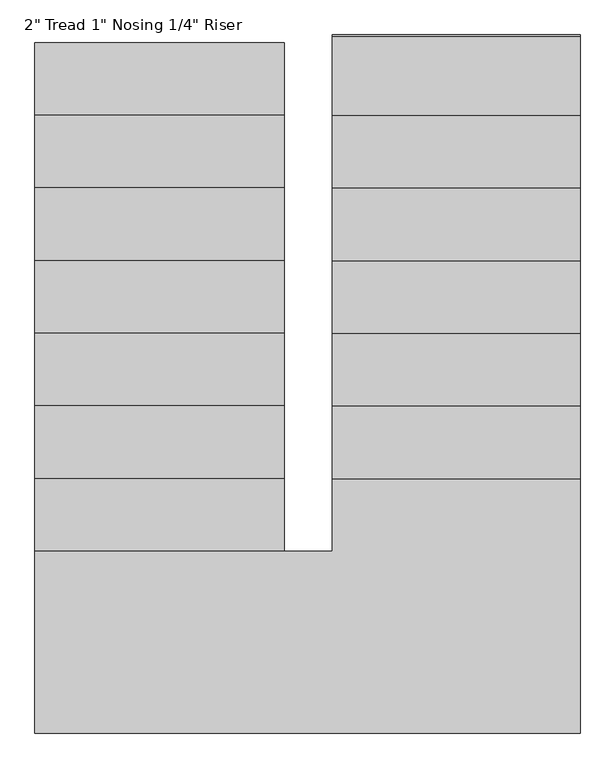
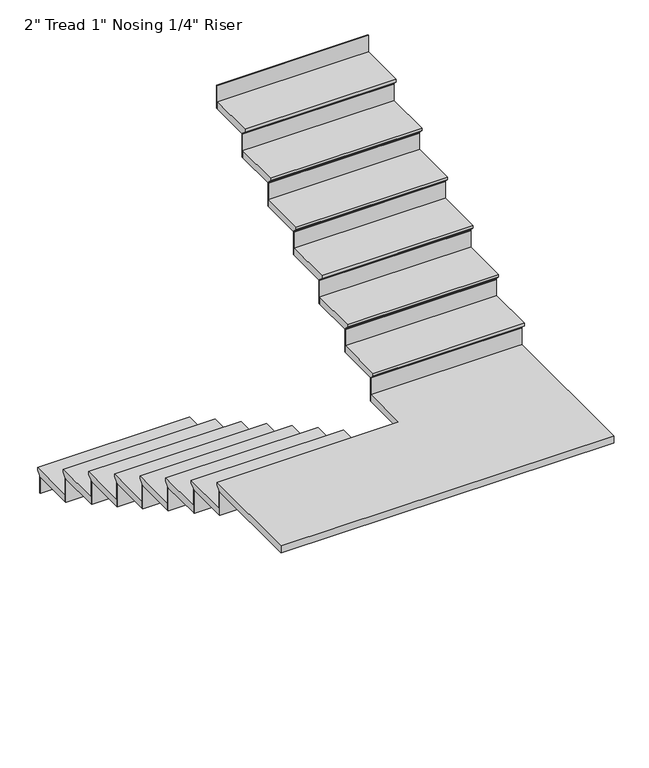
"""IFC4 building model written with IfcOpenShell, lengths in millimetres: stair flight geometry."""

from ifc_helpers import new_model, si_unit, origin, place, context, project, spatial, faceted_brep, source, transform, mapped, element, save


def stair_flight_bd25c6f5(model_context):
    return source(origin(), model_context, "Body", "Brep", [
        faceted_brep([(-4232.280864, -3571.6080018, 12799.4833333), (-4232.280864, -3571.6080018, 12818.5333333), (-3187.6083919, -3571.6080018, 12818.5333333), (-3187.6083919, -3571.6080018, 12799.4833333), (-4232.280864, -3597.0080018, 12774.0833333), (-3187.6083919, -3597.0080018, 12774.0833333), (-4232.280864, -3901.8080018, 12818.5333333), (-3187.6083919, -3901.8080018, 12818.5333333), (-3187.6083919, -3597.0080018, 12767.7333333), (-3187.6083919, -3901.8080018, 12767.7333333), (-4232.280864, -3901.8080018, 12767.7333333), (-4232.280864, -3597.0080018, 12767.7333333)], [[[0, 1, 2, 3]], [[4, 0, 3, 5]], [[2, 1, 6, 7]], [[8, 9, 10, 11]], [[2, 7, 9, 8, 5, 3]], [[8, 11, 4, 5]], [[6, 1, 0, 4, 11, 10]], [[7, 6, 10, 9]]]),
        faceted_brep([(-4232.280864, -3597.0080018, 12767.7333333), (-4232.280864, -3597.0080018, 12649.2), (-4232.280864, -3603.3580018, 12649.2), (-4232.280864, -3603.3580018, 12767.7333333), (-3187.6083919, -3597.0080018, 12767.7333333), (-3187.6083919, -3603.3580018, 12767.7333333), (-3187.6083919, -3603.3580018, 12649.2), (-3187.6083919, -3597.0080018, 12649.2)], [[[0, 1, 2, 3]], [[4, 5, 6, 7]], [[1, 0, 4, 7]], [[2, 1, 7, 6]], [[3, 2, 6, 5]], [[0, 3, 5, 4]]]),
        faceted_brep([(-4232.280864, -3901.8080018, 12937.0666667), (-4232.280864, -3901.8080018, 12767.7333333), (-4232.280864, -3908.1580018, 12767.7333333), (-4232.280864, -3908.1580018, 12937.0666667), (-3187.6083919, -3901.8080018, 12937.0666667), (-3187.6083919, -3908.1580018, 12937.0666667), (-3187.6083919, -3908.1580018, 12767.7333333), (-3187.6083919, -3901.8080018, 12767.7333333)], [[[0, 1, 2, 3]], [[4, 5, 6, 7]], [[1, 0, 4, 7]], [[2, 1, 7, 6]], [[3, 2, 6, 5]], [[0, 3, 5, 4]]]),
        faceted_brep([(-3187.6083919, -3876.4080018, 12987.8666667), (-4232.280864, -3876.4080018, 12987.8666667), (-4232.280864, -4206.6080018, 12987.8666667), (-3187.6083919, -4206.6080018, 12987.8666667), (-3187.6083919, -3901.8080018, 12937.0666667), (-3187.6083919, -4206.6080018, 12937.0666667), (-4232.280864, -4206.6080018, 12937.0666667), (-4232.280864, -3901.8080018, 12937.0666667), (-3187.6083919, -3901.8080018, 12943.4166667), (-3187.6083919, -3876.4080018, 12968.8166667), (-4232.280864, -3901.8080018, 12943.4166667), (-4232.280864, -3876.4080018, 12968.8166667)], [[[0, 1, 2, 3]], [[4, 5, 6, 7]], [[0, 3, 5, 4, 8, 9]], [[4, 7, 10, 8]], [[2, 1, 11, 10, 7, 6]], [[3, 2, 6, 5]], [[11, 1, 0, 9]], [[10, 11, 9, 8]]]),
        faceted_brep([(-4232.280864, -4206.6080018, 13106.4), (-4232.280864, -4206.6080018, 12937.0666667), (-4232.280864, -4212.9580018, 12937.0666667), (-4232.280864, -4212.9580018, 13106.4), (-3187.6083919, -4206.6080018, 13106.4), (-3187.6083919, -4212.9580018, 13106.4), (-3187.6083919, -4212.9580018, 12937.0666667), (-3187.6083919, -4206.6080018, 12937.0666667)], [[[0, 1, 2, 3]], [[4, 5, 6, 7]], [[1, 0, 4, 7]], [[2, 1, 7, 6]], [[3, 2, 6, 5]], [[0, 3, 5, 4]]]),
        faceted_brep([(-3187.6083919, -4181.2080018, 13157.2), (-4232.280864, -4181.2080018, 13157.2), (-4232.280864, -4511.4080018, 13157.2), (-3187.6083919, -4511.4080018, 13157.2), (-3187.6083919, -4206.6080018, 13106.4), (-3187.6083919, -4511.4080018, 13106.4), (-4232.280864, -4511.4080018, 13106.4), (-4232.280864, -4206.6080018, 13106.4), (-3187.6083919, -4206.6080018, 13112.75), (-3187.6083919, -4181.2080018, 13138.15), (-4232.280864, -4206.6080018, 13112.75), (-4232.280864, -4181.2080018, 13138.15)], [[[0, 1, 2, 3]], [[4, 5, 6, 7]], [[0, 3, 5, 4, 8, 9]], [[4, 7, 10, 8]], [[2, 1, 11, 10, 7, 6]], [[3, 2, 6, 5]], [[11, 1, 0, 9]], [[10, 11, 9, 8]]]),
        faceted_brep([(-4232.280864, -4511.4080018, 13275.7333333), (-4232.280864, -4511.4080018, 13106.4), (-4232.280864, -4517.7580018, 13106.4), (-4232.280864, -4517.7580018, 13275.7333333), (-3187.6083919, -4511.4080018, 13275.7333333), (-3187.6083919, -4517.7580018, 13275.7333333), (-3187.6083919, -4517.7580018, 13106.4), (-3187.6083919, -4511.4080018, 13106.4)], [[[0, 1, 2, 3]], [[4, 5, 6, 7]], [[1, 0, 4, 7]], [[2, 1, 7, 6]], [[3, 2, 6, 5]], [[0, 3, 5, 4]]]),
        faceted_brep([(-3187.6083919, -4486.0080018, 13326.5333333), (-4232.280864, -4486.0080018, 13326.5333333), (-4232.280864, -4816.2080018, 13326.5333333), (-3187.6083919, -4816.2080018, 13326.5333333), (-3187.6083919, -4511.4080018, 13275.7333333), (-3187.6083919, -4816.2080018, 13275.7333333), (-4232.280864, -4816.2080018, 13275.7333333), (-4232.280864, -4511.4080018, 13275.7333333), (-3187.6083919, -4511.4080018, 13282.0833333), (-3187.6083919, -4486.0080018, 13307.4833333), (-4232.280864, -4511.4080018, 13282.0833333), (-4232.280864, -4486.0080018, 13307.4833333)], [[[0, 1, 2, 3]], [[4, 5, 6, 7]], [[0, 3, 5, 4, 8, 9]], [[4, 7, 10, 8]], [[2, 1, 11, 10, 7, 6]], [[3, 2, 6, 5]], [[11, 1, 0, 9]], [[10, 11, 9, 8]]]),
        faceted_brep([(-4232.280864, -4816.2080018, 13445.0666667), (-4232.280864, -4816.2080018, 13275.7333333), (-4232.280864, -4822.5580018, 13275.7333333), (-4232.280864, -4822.5580018, 13445.0666667), (-3187.6083919, -4816.2080018, 13445.0666667), (-3187.6083919, -4822.5580018, 13445.0666667), (-3187.6083919, -4822.5580018, 13275.7333333), (-3187.6083919, -4816.2080018, 13275.7333333)], [[[0, 1, 2, 3]], [[4, 5, 6, 7]], [[1, 0, 4, 7]], [[2, 1, 7, 6]], [[3, 2, 6, 5]], [[0, 3, 5, 4]]]),
        faceted_brep([(-3187.6083919, -4790.8080018, 13495.8666667), (-4232.280864, -4790.8080018, 13495.8666667), (-4232.280864, -5121.0080018, 13495.8666667), (-3187.6083919, -5121.0080018, 13495.8666667), (-3187.6083919, -4816.2080018, 13445.0666667), (-3187.6083919, -5121.0080018, 13445.0666667), (-4232.280864, -5121.0080018, 13445.0666667), (-4232.280864, -4816.2080018, 13445.0666667), (-3187.6083919, -4816.2080018, 13451.4166667), (-3187.6083919, -4790.8080018, 13476.8166667), (-4232.280864, -4816.2080018, 13451.4166667), (-4232.280864, -4790.8080018, 13476.8166667)], [[[0, 1, 2, 3]], [[4, 5, 6, 7]], [[0, 3, 5, 4, 8, 9]], [[4, 7, 10, 8]], [[2, 1, 11, 10, 7, 6]], [[3, 2, 6, 5]], [[11, 1, 0, 9]], [[10, 11, 9, 8]]]),
        faceted_brep([(-4232.280864, -5121.0080018, 13614.4), (-4232.280864, -5121.0080018, 13445.0666667), (-4232.280864, -5127.3580018, 13445.0666667), (-4232.280864, -5127.3580018, 13614.4), (-3187.6083919, -5121.0080018, 13614.4), (-3187.6083919, -5127.3580018, 13614.4), (-3187.6083919, -5127.3580018, 13445.0666667), (-3187.6083919, -5121.0080018, 13445.0666667)], [[[0, 1, 2, 3]], [[4, 5, 6, 7]], [[1, 0, 4, 7]], [[2, 1, 7, 6]], [[3, 2, 6, 5]], [[0, 3, 5, 4]]]),
        faceted_brep([(-3187.6083919, -5095.6080018, 13665.2), (-4232.280864, -5095.6080018, 13665.2), (-4232.280864, -5425.8080018, 13665.2), (-3187.6083919, -5425.8080018, 13665.2), (-3187.6083919, -5121.0080018, 13614.4), (-3187.6083919, -5425.8080018, 13614.4), (-4232.280864, -5425.8080018, 13614.4), (-4232.280864, -5121.0080018, 13614.4), (-3187.6083919, -5121.0080018, 13620.75), (-3187.6083919, -5095.6080018, 13646.15), (-4232.280864, -5121.0080018, 13620.75), (-4232.280864, -5095.6080018, 13646.15)], [[[0, 1, 2, 3]], [[4, 5, 6, 7]], [[0, 3, 5, 4, 8, 9]], [[4, 7, 10, 8]], [[2, 1, 11, 10, 7, 6]], [[3, 2, 6, 5]], [[11, 1, 0, 9]], [[10, 11, 9, 8]]]),
        faceted_brep([(-4232.280864, -5425.8080018, 13783.7333333), (-4232.280864, -5425.8080018, 13614.4), (-4232.280864, -5432.1580018, 13614.4), (-4232.280864, -5432.1580018, 13783.7333333), (-3187.6083919, -5425.8080018, 13783.7333333), (-3187.6083919, -5432.1580018, 13783.7333333), (-3187.6083919, -5432.1580018, 13614.4), (-3187.6083919, -5425.8080018, 13614.4)], [[[0, 1, 2, 3]], [[4, 5, 6, 7]], [[1, 0, 4, 7]], [[2, 1, 7, 6]], [[3, 2, 6, 5]], [[0, 3, 5, 4]]]),
        faceted_brep([(-3187.6083919, -5400.4080018, 13834.5333333), (-4232.280864, -5400.4080018, 13834.5333333), (-4232.280864, -5730.6080018, 13834.5333333), (-3187.6083919, -5730.6080018, 13834.5333333), (-3187.6083919, -5425.8080018, 13783.7333333), (-3187.6083919, -5730.6080018, 13783.7333333), (-4232.280864, -5730.6080018, 13783.7333333), (-4232.280864, -5425.8080018, 13783.7333333), (-3187.6083919, -5425.8080018, 13790.0833333), (-3187.6083919, -5400.4080018, 13815.4833333), (-4232.280864, -5425.8080018, 13790.0833333), (-4232.280864, -5400.4080018, 13815.4833333)], [[[0, 1, 2, 3]], [[4, 5, 6, 7]], [[0, 3, 5, 4, 8, 9]], [[4, 7, 10, 8]], [[2, 1, 11, 10, 7, 6]], [[3, 2, 6, 5]], [[11, 1, 0, 9]], [[10, 11, 9, 8]]]),
        faceted_brep([(-4232.280864, -5730.6080018, 13953.0666667), (-4232.280864, -5730.6080018, 13783.7333333), (-4232.280864, -5736.9580018, 13783.7333333), (-4232.280864, -5736.9580018, 13953.0666667), (-3187.6083919, -5730.6080018, 13953.0666667), (-3187.6083919, -5736.9580018, 13953.0666667), (-3187.6083919, -5736.9580018, 13783.7333333), (-3187.6083919, -5730.6080018, 13783.7333333)], [[[0, 1, 2, 3]], [[4, 5, 6, 7]], [[1, 0, 4, 7]], [[2, 1, 7, 6]], [[3, 2, 6, 5]], [[0, 3, 5, 4]]]),
        faceted_brep([(-2984.4083919, -5375.0080018, 14003.8666667), (-2984.4083919, -5705.2080018, 14003.8666667), (-4232.280864, -5705.2080018, 14003.8666667), (-4232.280864, -6467.2080018, 14003.8666667), (-1946.280864, -6467.2080018, 14003.8666667), (-1946.280864, -5375.0080018, 14003.8666667), (-2984.4083919, -5705.2080018, 13953.0666667), (-2984.4083919, -5375.0080018, 13953.0666667), (-1946.280864, -5375.0080018, 13953.0666667), (-1946.280864, -6467.2080018, 13953.0666667), (-4232.280864, -6467.2080018, 13953.0666667), (-4232.280864, -5730.6080018, 13953.0666667), (-3187.6083919, -5730.6080018, 13953.0666667), (-3187.6083919, -5705.2080018, 13953.0666667), (-3187.6083919, -5705.2080018, 13984.8166667), (-4232.280864, -5705.2080018, 13984.8166667), (-3187.6083919, -5730.6080018, 13959.4166667), (-4232.280864, -5730.6080018, 13959.4166667)], [[[0, 1, 2, 3, 4, 5]], [[6, 7, 8, 9, 10, 11, 12, 13]], [[1, 0, 7, 6]], [[2, 1, 6, 13, 14, 15]], [[13, 12, 16, 14]], [[12, 11, 17, 16]], [[3, 2, 15, 17, 11, 10]], [[4, 3, 10, 9]], [[5, 4, 9, 8]], [[0, 5, 8, 7]], [[17, 15, 14, 16]]]),
        faceted_brep([(-1946.280864, -5375.0080018, 14122.4), (-1946.280864, -5375.0080018, 13953.0666667), (-1946.280864, -5368.6580018, 13953.0666667), (-1946.280864, -5368.6580018, 14122.4), (-2984.4083919, -5375.0080018, 14122.4), (-2984.4083919, -5368.6580018, 14122.4), (-2984.4083919, -5368.6580018, 13953.0666667), (-2984.4083919, -5375.0080018, 13953.0666667)], [[[0, 1, 2, 3]], [[4, 5, 6, 7]], [[1, 0, 4, 7]], [[2, 1, 7, 6]], [[3, 2, 6, 5]], [[0, 3, 5, 4]]]),
        faceted_brep([(-2984.4083919, -5400.4080018, 14173.2), (-1946.280864, -5400.4080018, 14173.2), (-1946.280864, -5070.2080018, 14173.2), (-2984.4083919, -5070.2080018, 14173.2), (-2984.4083919, -5375.0080018, 14122.4), (-2984.4083919, -5070.2080018, 14122.4), (-1946.280864, -5070.2080018, 14122.4), (-1946.280864, -5375.0080018, 14122.4), (-2984.4083919, -5375.0080018, 14128.75), (-2984.4083919, -5400.4080018, 14154.15), (-1946.280864, -5375.0080018, 14128.75), (-1946.280864, -5400.4080018, 14154.15)], [[[0, 1, 2, 3]], [[4, 5, 6, 7]], [[0, 3, 5, 4, 8, 9]], [[4, 7, 10, 8]], [[2, 1, 11, 10, 7, 6]], [[3, 2, 6, 5]], [[11, 1, 0, 9]], [[10, 11, 9, 8]]]),
        faceted_brep([(-1946.280864, -5070.2080018, 14291.7333333), (-1946.280864, -5070.2080018, 14122.4), (-1946.280864, -5063.8580018, 14122.4), (-1946.280864, -5063.8580018, 14291.7333333), (-2984.4083919, -5070.2080018, 14291.7333333), (-2984.4083919, -5063.8580018, 14291.7333333), (-2984.4083919, -5063.8580018, 14122.4), (-2984.4083919, -5070.2080018, 14122.4)], [[[0, 1, 2, 3]], [[4, 5, 6, 7]], [[1, 0, 4, 7]], [[2, 1, 7, 6]], [[3, 2, 6, 5]], [[0, 3, 5, 4]]]),
        faceted_brep([(-2984.4083919, -5095.6080018, 14342.5333333), (-1946.280864, -5095.6080018, 14342.5333333), (-1946.280864, -4765.4080018, 14342.5333333), (-2984.4083919, -4765.4080018, 14342.5333333), (-2984.4083919, -5070.2080018, 14291.7333333), (-2984.4083919, -4765.4080018, 14291.7333333), (-1946.280864, -4765.4080018, 14291.7333333), (-1946.280864, -5070.2080018, 14291.7333333), (-2984.4083919, -5070.2080018, 14298.0833333), (-2984.4083919, -5095.6080018, 14323.4833333), (-1946.280864, -5070.2080018, 14298.0833333), (-1946.280864, -5095.6080018, 14323.4833333)], [[[0, 1, 2, 3]], [[4, 5, 6, 7]], [[0, 3, 5, 4, 8, 9]], [[4, 7, 10, 8]], [[2, 1, 11, 10, 7, 6]], [[3, 2, 6, 5]], [[11, 1, 0, 9]], [[10, 11, 9, 8]]]),
        faceted_brep([(-1946.280864, -4765.4080018, 14461.0666667), (-1946.280864, -4765.4080018, 14291.7333333), (-1946.280864, -4759.0580018, 14291.7333333), (-1946.280864, -4759.0580018, 14461.0666667), (-2984.4083919, -4765.4080018, 14461.0666667), (-2984.4083919, -4759.0580018, 14461.0666667), (-2984.4083919, -4759.0580018, 14291.7333333), (-2984.4083919, -4765.4080018, 14291.7333333)], [[[0, 1, 2, 3]], [[4, 5, 6, 7]], [[1, 0, 4, 7]], [[2, 1, 7, 6]], [[3, 2, 6, 5]], [[0, 3, 5, 4]]]),
        faceted_brep([(-2984.4083919, -4790.8080018, 14511.8666667), (-1946.280864, -4790.8080018, 14511.8666667), (-1946.280864, -4460.6080018, 14511.8666667), (-2984.4083919, -4460.6080018, 14511.8666667), (-2984.4083919, -4765.4080018, 14461.0666667), (-2984.4083919, -4460.6080018, 14461.0666667), (-1946.280864, -4460.6080018, 14461.0666667), (-1946.280864, -4765.4080018, 14461.0666667), (-2984.4083919, -4765.4080018, 14467.4166667), (-2984.4083919, -4790.8080018, 14492.8166667), (-1946.280864, -4765.4080018, 14467.4166667), (-1946.280864, -4790.8080018, 14492.8166667)], [[[0, 1, 2, 3]], [[4, 5, 6, 7]], [[0, 3, 5, 4, 8, 9]], [[4, 7, 10, 8]], [[2, 1, 11, 10, 7, 6]], [[3, 2, 6, 5]], [[11, 1, 0, 9]], [[10, 11, 9, 8]]]),
        faceted_brep([(-1946.280864, -4460.6080018, 14630.4), (-1946.280864, -4460.6080018, 14461.0666667), (-1946.280864, -4454.2580018, 14461.0666667), (-1946.280864, -4454.2580018, 14630.4), (-2984.4083919, -4460.6080018, 14630.4), (-2984.4083919, -4454.2580018, 14630.4), (-2984.4083919, -4454.2580018, 14461.0666667), (-2984.4083919, -4460.6080018, 14461.0666667)], [[[0, 1, 2, 3]], [[4, 5, 6, 7]], [[1, 0, 4, 7]], [[2, 1, 7, 6]], [[3, 2, 6, 5]], [[0, 3, 5, 4]]]),
        faceted_brep([(-2984.4083919, -4486.0080018, 14681.2), (-1946.280864, -4486.0080018, 14681.2), (-1946.280864, -4155.8080018, 14681.2), (-2984.4083919, -4155.8080018, 14681.2), (-2984.4083919, -4460.6080018, 14630.4), (-2984.4083919, -4155.8080018, 14630.4), (-1946.280864, -4155.8080018, 14630.4), (-1946.280864, -4460.6080018, 14630.4), (-2984.4083919, -4460.6080018, 14636.75), (-2984.4083919, -4486.0080018, 14662.15), (-1946.280864, -4460.6080018, 14636.75), (-1946.280864, -4486.0080018, 14662.15)], [[[0, 1, 2, 3]], [[4, 5, 6, 7]], [[0, 3, 5, 4, 8, 9]], [[4, 7, 10, 8]], [[2, 1, 11, 10, 7, 6]], [[3, 2, 6, 5]], [[11, 1, 0, 9]], [[10, 11, 9, 8]]]),
        faceted_brep([(-1946.280864, -4155.8080018, 14799.7333333), (-1946.280864, -4155.8080018, 14630.4), (-1946.280864, -4149.4580018, 14630.4), (-1946.280864, -4149.4580018, 14799.7333333), (-2984.4083919, -4155.8080018, 14799.7333333), (-2984.4083919, -4149.4580018, 14799.7333333), (-2984.4083919, -4149.4580018, 14630.4), (-2984.4083919, -4155.8080018, 14630.4)], [[[0, 1, 2, 3]], [[4, 5, 6, 7]], [[1, 0, 4, 7]], [[2, 1, 7, 6]], [[3, 2, 6, 5]], [[0, 3, 5, 4]]]),
        faceted_brep([(-2984.4083919, -4181.2080018, 14850.5333333), (-1946.280864, -4181.2080018, 14850.5333333), (-1946.280864, -3851.0080018, 14850.5333333), (-2984.4083919, -3851.0080018, 14850.5333333), (-2984.4083919, -4155.8080018, 14799.7333333), (-2984.4083919, -3851.0080018, 14799.7333333), (-1946.280864, -3851.0080018, 14799.7333333), (-1946.280864, -4155.8080018, 14799.7333333), (-2984.4083919, -4155.8080018, 14806.0833333), (-2984.4083919, -4181.2080018, 14831.4833333), (-1946.280864, -4155.8080018, 14806.0833333), (-1946.280864, -4181.2080018, 14831.4833333)], [[[0, 1, 2, 3]], [[4, 5, 6, 7]], [[0, 3, 5, 4, 8, 9]], [[4, 7, 10, 8]], [[2, 1, 11, 10, 7, 6]], [[3, 2, 6, 5]], [[11, 1, 0, 9]], [[10, 11, 9, 8]]]),
        faceted_brep([(-1946.280864, -3851.0080018, 14969.0666667), (-1946.280864, -3851.0080018, 14799.7333333), (-1946.280864, -3844.6580018, 14799.7333333), (-1946.280864, -3844.6580018, 14969.0666667), (-2984.4083919, -3851.0080018, 14969.0666667), (-2984.4083919, -3844.6580018, 14969.0666667), (-2984.4083919, -3844.6580018, 14799.7333333), (-2984.4083919, -3851.0080018, 14799.7333333)], [[[0, 1, 2, 3]], [[4, 5, 6, 7]], [[1, 0, 4, 7]], [[2, 1, 7, 6]], [[3, 2, 6, 5]], [[0, 3, 5, 4]]]),
        faceted_brep([(-1946.280864, -3546.2080018, 15138.4), (-1946.280864, -3546.2080018, 14969.0666667), (-1946.280864, -3539.8580018, 14969.0666667), (-1946.280864, -3539.8580018, 15138.4), (-2984.4083919, -3546.2080018, 15138.4), (-2984.4083919, -3539.8580018, 15138.4), (-2984.4083919, -3539.8580018, 14969.0666667), (-2984.4083919, -3546.2080018, 14969.0666667)], [[[0, 1, 2, 3]], [[4, 5, 6, 7]], [[1, 0, 4, 7]], [[2, 1, 7, 6]], [[3, 2, 6, 5]], [[0, 3, 5, 4]]]),
        faceted_brep([(-2984.4083919, -3876.4080018, 15019.8666667), (-1946.280864, -3876.4080018, 15019.8666667), (-1946.280864, -3546.2080018, 15019.8666667), (-2984.4083919, -3546.2080018, 15019.8666667), (-2984.4083919, -3851.0080018, 14969.0666667), (-2984.4083919, -3546.2080018, 14969.0666667), (-1946.280864, -3546.2080018, 14969.0666667), (-1946.280864, -3851.0080018, 14969.0666667), (-2984.4083919, -3851.0080018, 14975.4166667), (-2984.4083919, -3876.4080018, 15000.8166667), (-1946.280864, -3851.0080018, 14975.4166667), (-1946.280864, -3876.4080018, 15000.8166667)], [[[0, 1, 2, 3]], [[4, 5, 6, 7]], [[0, 3, 5, 4, 8, 9]], [[4, 7, 10, 8]], [[2, 1, 11, 10, 7, 6]], [[3, 2, 6, 5]], [[11, 1, 0, 9]], [[10, 11, 9, 8]]]),
    ])


if __name__ == "__main__":
    model = new_model("IFC4")
    model_context = context("Model", 3, world=origin())
    ifc_project = project(units=[si_unit("LENGTHUNIT", "METRE", prefix="MILLI")], contexts=[model_context])
    site = spatial("IfcSite", under=ifc_project)
    building = spatial("IfcBuilding", under=site)
    placement = place(None, origin())
    stair_flight_shape = stair_flight_bd25c6f5(model_context)
    element("IfcStairFlight", 1, ObjectType="2\" Tread 1\" Nosing 1/4\" Riser", at=placement, inside=building, context=model_context, shape_type="MappedRepresentation", body=[
        mapped(stair_flight_shape, transform((0.0, 0.0, 0.0), x_axis=(1.0, 0.0, 0.0), y_axis=(0.0, 1.0, 0.0), z_axis=(0.0, 0.0, 1.0))),
    ])
    save(model, "model.ifc")
